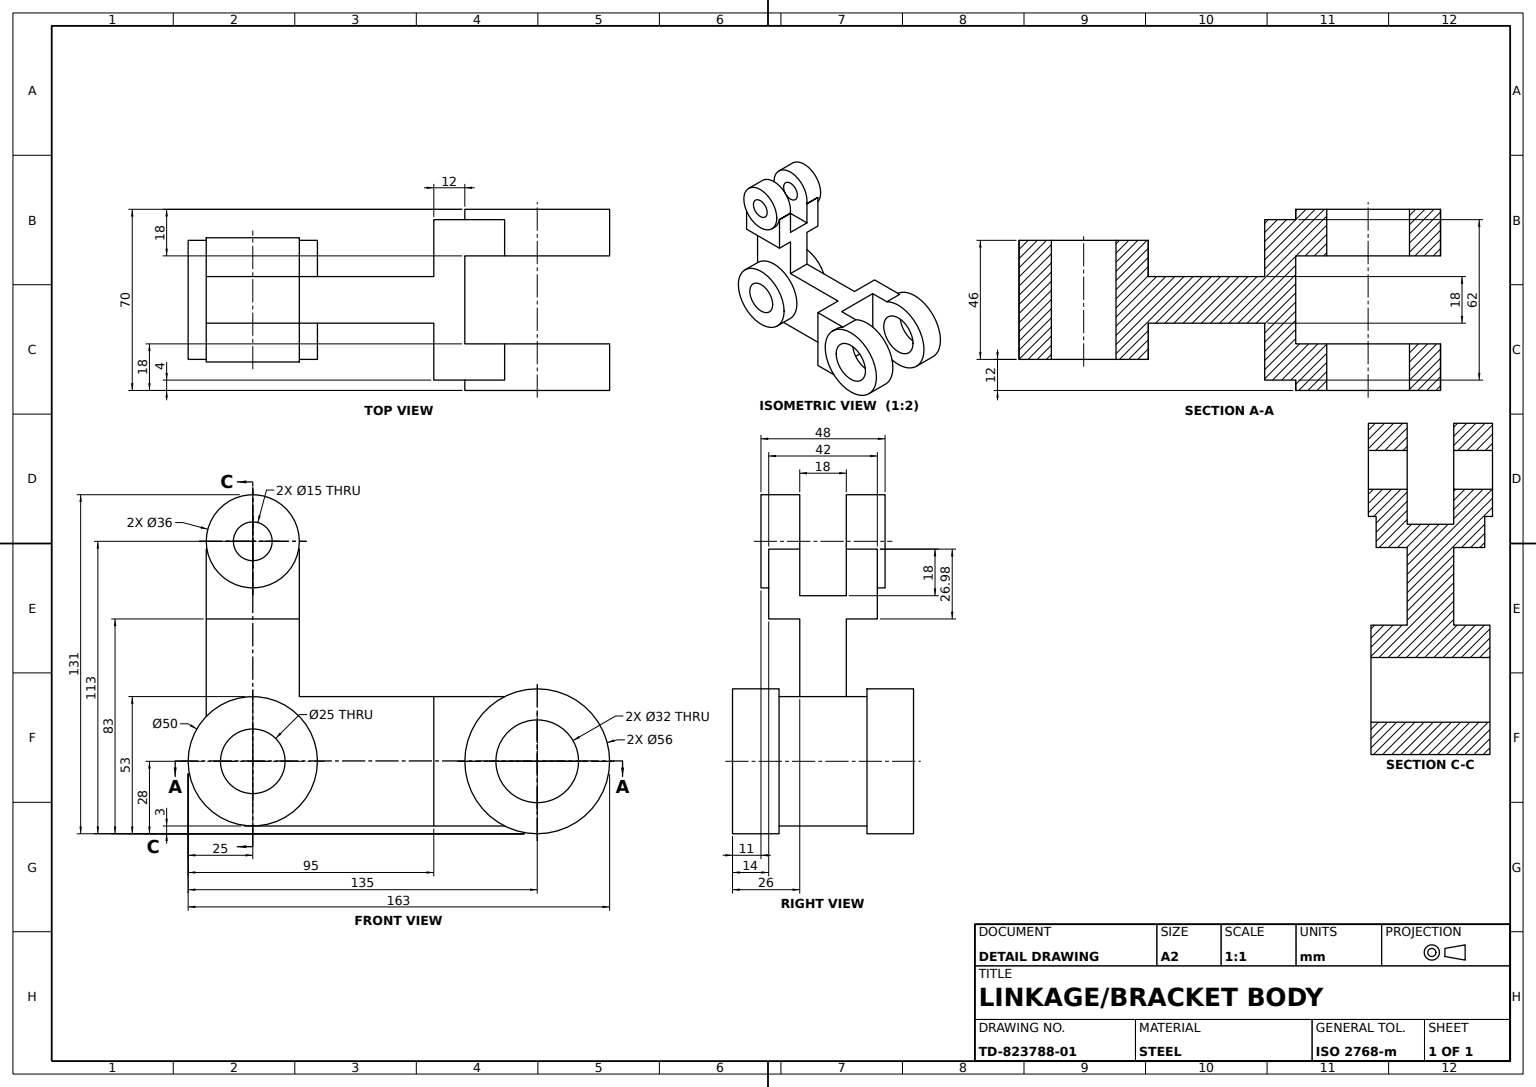
from build123d import *

# Parameters (mm, degrees)
BASE_PLATE_DEPTH                = 12
EYE_BOSS_A_SKETCH_R             = 28
EYE_BOSS_A_56_DEPTH             = 14
EYE_HUB_A_SKETCH_R              = 28
EYE_HUB_A_56X4_DEPTH            = 4
EYE_WEB_A_DEPTH                 = 14
EYE_START                       = -14
EYE_BOSS_B_SKETCH_R             = 28
EYE_BOSS_B_DEPTH                = 14
EYE_HUB_B_SKETCH_R              = 28
EYE_HUB_B_56X4_DEPTH            = 4
SIDE_BOSS_SKETCH_R              = 25
SIDE_BOSS_50_DEPTH              = 62
SIDE_BOSS_FACE_CUT_A_SKETCH_R   = 25
SIDE_BOSS_FACE_CUT_A_50X8_DEPTH = 8
SIDE_BOSS_FACE_CUT_B_SKETCH_R   = 25
SIDE_BOSS_FACE_CUT_B_50X8_DEPTH = 8
SIDE_BORE_SKETCH_R              = 12.5
SIDE_BORE_25_DEPTH              = 46
EYE_BORE_SKETCH_R               = 16
EYE_BORE_32_DEPTH               = 80
CENTRAL_BODY_DEPTH              = 50
BODY_START                      = -50
BODY_SLOT_CUT_DEPTH             = 50
UPPER_LUG_A_SKETCH_R            = 18
UPPER_LUG_A_36_DEPTH            = 15
UPPER_LUG_B_SKETCH_R            = 18
UPPER_LUG_B_36_DEPTH            = 15
UPPER_CLEVIS_BODY_DEPTH         = 36
UPPER_CLEVIS_INFILL_SKETCH_W    = 18
UPPER_CLEVIS_INFILL_SKETCH_H    = 12
UPPER_CLEVIS_INFILL_DEPTH       = 36
CLEVIS_SLOT_A_SKETCH_W          = 36
CLEVIS_SLOT_A_SKETCH_H          = 18
CLEVIS_SLOT_A_DEPTH             = 12
CLEVIS_SLOT_B_SKETCH_W          = 36
CLEVIS_SLOT_B_SKETCH_H          = 18
CLEVIS_SLOT_B_DEPTH             = 12
LUG_PIN_HOLE_SKETCH_R           = 7.5
LUG_PIN_HOLE_15_DEPTH           = 60
SIDE_SLOT_CUT_DEPTH             = 60


with BuildPart() as part:
    # Base Plate Sketch → Base Plate (new body)
    with BuildSketch(Plane.XY):
        Polygon((0, 0), (14, 0), (48, 0), (62, 0), (62, 50), (0, 50), align=None)
    extrude(amount=BASE_PLATE_DEPTH)



with BuildPart() as body_2:
    # Eye Boss A Sketch → Eye Boss A _56 (new body)
    with BuildSketch(Plane(origin=(62, 0, 0), x_dir=(0, 0, -1), z_dir=(1, 0, 0))):
        with Locations((28, 25)):
            Circle(EYE_BOSS_A_SKETCH_R)
    extrude(amount=-EYE_BOSS_A_56_DEPTH)

    # Eye Hub A Sketch → Eye Hub A _56x4 (add)
    with BuildSketch(Plane(origin=(62, 0, 0), x_dir=(0, 0, -1), z_dir=(1, 0, 0))):
        with Locations((28, 25)):
            Circle(EYE_HUB_A_SKETCH_R)
    extrude(amount=EYE_HUB_A_56X4_DEPTH)


with BuildPart() as part_1:
    add(part.part)

    add(body_2.part)  # Eye Web A merges body 2
    # Eye Web A Sketch → Eye Web A (add)
    with BuildSketch(Plane(origin=(62, 0, 0), x_dir=(0, 0, -1), z_dir=(1, 0, 0))):
        with BuildLine():
            Line((15.390479787, 50), (0, 50))
            Line((0, 50), (0, 25.000000117))
            ThreePointArc((0, 25.000000117), (4.156064051, 39.678784639), (15.390479787, 50))
        make_face()
        with BuildLine():
            ThreePointArc((15.390479787, 0), (4.15606399, 10.32121546), (0, 25.000000117))
            Line((0, 25.000000117), (0, 0))
            Line((0, 0), (15.390479787, 0))
        make_face()
    extrude(amount=-EYE_WEB_A_DEPTH)

    # Eye Boss B Sketch → Eye Boss B (add)
    with BuildSketch(Plane.ZY.offset(EYE_START)):
        with Locations(Location((-28, 25, 0), (0, 0, 180))):
            Circle(EYE_BOSS_B_SKETCH_R)
        with BuildLine():
            Line((0, 25), (0, 50))
            Line((0, 50), (-15.390479787, 50))
            ThreePointArc((-15.390479787, 50), (-4.156064021, 39.678784589), (0, 25))
        make_face()
        with BuildLine():
            Line((0, 0), (0, 25))
            ThreePointArc((0, 25), (-4.156064021, 10.321215411), (-15.390479787, 0))
            Line((-15.390479787, 0), (0, 0))
        make_face()
    extrude(amount=EYE_BOSS_B_DEPTH)

    # Eye Hub B Sketch → Eye Hub B _56x4 (add)
    with BuildSketch(Plane.ZY):
        with Locations(Location((-28, 25, 0), (0, 0, 180))):
            Circle(EYE_HUB_B_SKETCH_R)
    extrude(amount=EYE_HUB_B_56X4_DEPTH)

    # Eye Bore Sketch → Eye Bore _32 (cut)
    with BuildSketch(Plane(origin=(66, 0, 0), x_dir=(0, 0, -1), z_dir=(1, 0, 0))):
        with Locations(Location((28, 25, 0), (0, 0, 180))):
            Circle(EYE_BORE_SKETCH_R)
    extrude(amount=-EYE_BORE_32_DEPTH, mode=Mode.SUBTRACT)



with BuildPart() as body_2_2:
    # Side Boss Sketch → Side Boss _50 (new body)
    with BuildSketch(Plane(origin=(62, 0, 0), x_dir=(0, 0, -1), z_dir=(1, 0, 0))):
        with Locations((-82, 25)):
            Circle(SIDE_BOSS_SKETCH_R)
    extrude(amount=-SIDE_BOSS_50_DEPTH)

    # Side Boss Face Cut A Sketch → Side Boss Face Cut A _50x8 (cut)
    with BuildSketch(Plane(origin=(62, 0, 0), x_dir=(0, 0, -1), z_dir=(1, 0, 0))):
        with Locations((-82, 25)):
            Circle(SIDE_BOSS_FACE_CUT_A_SKETCH_R)
    extrude(amount=-SIDE_BOSS_FACE_CUT_A_50X8_DEPTH, mode=Mode.SUBTRACT)

    # Side Boss Face Cut B Sketch → Side Boss Face Cut B _50x8 (cut)
    with BuildSketch(Plane.ZY):
        with Locations(Location((82, 25, 0), (0, 0, 180))):
            Circle(SIDE_BOSS_FACE_CUT_B_SKETCH_R)
    extrude(amount=-SIDE_BOSS_FACE_CUT_B_50X8_DEPTH, mode=Mode.SUBTRACT)

    # Side Bore Sketch → Side Bore _25 (cut)
    with BuildSketch(Plane.ZY.offset(-8)):
        with Locations((82, 25)):
            Circle(SIDE_BORE_SKETCH_R)
    extrude(amount=-SIDE_BORE_25_DEPTH, mode=Mode.SUBTRACT)


with BuildPart() as part_2:
    add(part_1.part)

    add(body_2_2.part)  # Central Body merges body 2 2
    # Central Body Sketch → Central Body (add)
    with BuildSketch(Plane(origin=(0, 50, 0), x_dir=(1, 0, 0), z_dir=(0, 1, 0))):
        Polygon((31, -12), (22, -12), (22, -71.244384349), (22, -85.354634245), (40, -85.354634245), (40, -71.244384349), (40, -12), align=None)
    extrude(amount=-CENTRAL_BODY_DEPTH)

    # Body Slot Sketch → Body Slot Cut (cut)
    with BuildSketch(Plane(origin=(40, 0, 0), x_dir=(0, 0, -1), z_dir=(1, 0, 0)).offset(BODY_START)):
        with BuildLine():
            Line((-85.354634245, 37.041446303), (-85.354634245, 12.958553697))
            ThreePointArc((-85.354634245, 12.958553697), (-69.5, 25), (-85.354634245, 37.041446303))
        make_face()
    extrude(amount=BODY_SLOT_CUT_DEPTH, mode=Mode.SUBTRACT)



with BuildPart() as body_2_3:
    # Upper Lug A Sketch → Upper Lug A _36 (new body)
    with BuildSketch(Plane.ZY.offset(-22)):
        with Locations((82, 110)):
            Circle(UPPER_LUG_A_SKETCH_R)
    extrude(amount=UPPER_LUG_A_36_DEPTH)


with BuildPart() as body_3:
    # Upper Lug B Sketch → Upper Lug B _36 (new body)
    with BuildSketch(Plane(origin=(40, 0, 0), x_dir=(0, 0, -1), z_dir=(1, 0, 0))):
        with Locations((-82, 110)):
            Circle(UPPER_LUG_B_SKETCH_R)
    extrude(amount=UPPER_LUG_B_36_DEPTH)


with BuildPart() as part_3:
    add(part_2.part)

    add(body_2_3.part)  # Upper Clevis Body merges body 2 3

    add(body_3.part)  # Upper Clevis Body merges body 3
    # Upper Clevis Profile Sketch → Upper Clevis Body (add)
    with BuildSketch(Plane.XY.offset(100)):
        Polygon((22, 62), (22, 49.773906214), (22, 25.080522604), (40, 25.080522604), (40, 50), (40, 62), (52, 62), (52, 92), (52, 106.982899018), (40, 106.982899018), (40, 76.982899018), (22, 76.982899018), (22, 106.982899018), (10, 106.982899018), (10, 92), (10, 62), align=None)
    extrude(amount=-UPPER_CLEVIS_BODY_DEPTH)

    # Upper Clevis Infill Sketch → Upper Clevis Infill (add)
    with BuildSketch(Plane.XY.offset(100)):
        with Locations((31, 82.982899018)):
            Rectangle(UPPER_CLEVIS_INFILL_SKETCH_W, UPPER_CLEVIS_INFILL_SKETCH_H)
    extrude(amount=-UPPER_CLEVIS_INFILL_DEPTH)

    # Clevis Slot A Sketch → Clevis Slot A (cut)
    with BuildSketch(Plane(origin=(52, 0, 0), x_dir=(0, 0, -1), z_dir=(1, 0, 0))):
        with Locations((-82, 71)):
            Rectangle(CLEVIS_SLOT_A_SKETCH_W, CLEVIS_SLOT_A_SKETCH_H)
    extrude(amount=-CLEVIS_SLOT_A_DEPTH, mode=Mode.SUBTRACT)

    # Clevis Slot B Sketch → Clevis Slot B (cut)
    with BuildSketch(Plane.ZY.offset(-10)):
        with Locations((82, 71)):
            Rectangle(CLEVIS_SLOT_B_SKETCH_W, CLEVIS_SLOT_B_SKETCH_H)
    extrude(amount=-CLEVIS_SLOT_B_DEPTH, mode=Mode.SUBTRACT)

    # Lug Pin Hole Sketch → Lug Pin Hole _15 (cut)
    with BuildSketch(Plane(origin=(55, 0, 0), x_dir=(0, 0, -1), z_dir=(1, 0, 0))):
        with Locations((-82, 110)):
            Circle(LUG_PIN_HOLE_SKETCH_R)
    extrude(amount=-LUG_PIN_HOLE_15_DEPTH, mode=Mode.SUBTRACT)

    # Side Slot Sketch → Side Slot Cut (cut)
    with BuildSketch(Plane.ZY.offset(-22)):
        with BuildLine():
            Line((69.5, 25), (94.5, 25))
            ThreePointArc((94.5, 25), (82, 37.5), (69.5, 25))
        make_face()
    extrude(amount=-SIDE_SLOT_CUT_DEPTH, mode=Mode.SUBTRACT)


solid = part_3.part
